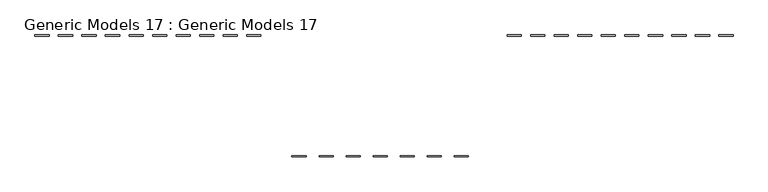
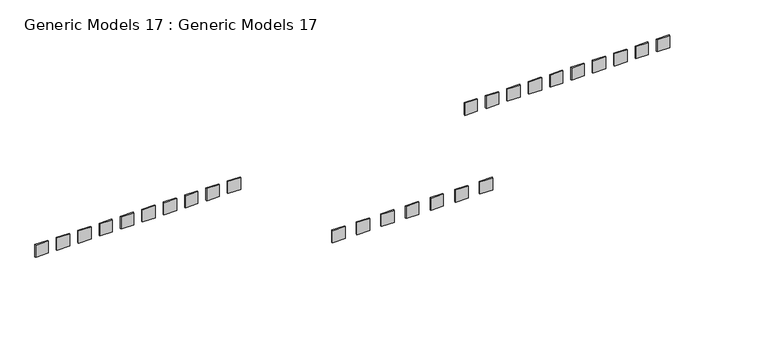
"""IFC4 building model written with IfcOpenShell, lengths in millimetres: proxy geometry, Generic Models 17 : Generic Models 17."""

from ifc_helpers import new_model, si_unit, frame, origin, place, context, project, spatial, polyline, outline, extrude, source, transform, mapped, element, save


def generic_models_17_generic_models_17_0ec560be(model_context):
    return source(origin(), model_context, "Body", "SweptSolid", [
        extrude(outline(polyline([(382.7174924, -8008.8292912), (77.9174924, -8008.8292912), (77.9174924, -7983.4292912), (382.7174924, -7983.4292912), (382.7174924, -8008.8292912)])), frame((0.0, 0.0, 6823.7646282), z_axis=(0.0, 0.0, 1.0), x_axis=(1.0, 0.0, 0.0)), (0.0, 0.0, 1.0), 304.8),
        extrude(outline(polyline([(-201.4825076, -8008.8292912), (-506.2825076, -8008.8292912), (-506.2825076, -7983.4292912), (-201.4825076, -7983.4292912), (-201.4825076, -8008.8292912)])), frame((0.0, 0.0, 6823.7646282), z_axis=(0.0, 0.0, 1.0), x_axis=(1.0, 0.0, 0.0)), (0.0, 0.0, 1.0), 304.8),
        extrude(outline(polyline([(-785.6825076, -8008.8292912), (-1090.4825076, -8008.8292912), (-1090.4825076, -7983.4292912), (-785.6825076, -7983.4292912), (-785.6825076, -8008.8292912)])), frame((0.0, 0.0, 6823.7646282), z_axis=(0.0, 0.0, 1.0), x_axis=(1.0, 0.0, 0.0)), (0.0, 0.0, 1.0), 304.8),
        extrude(outline(polyline([(-1369.8825076, -8008.8292912), (-1674.6825076, -8008.8292912), (-1674.6825076, -7983.4292912), (-1369.8825076, -7983.4292912), (-1369.8825076, -8008.8292912)])), frame((0.0, 0.0, 6823.7646282), z_axis=(0.0, 0.0, 1.0), x_axis=(1.0, 0.0, 0.0)), (0.0, 0.0, 1.0), 304.8),
        extrude(outline(polyline([(-1954.0825076, -8008.8292912), (-2258.8825076, -8008.8292912), (-2258.8825076, -7983.4292912), (-1954.0825076, -7983.4292912), (-1954.0825076, -8008.8292912)])), frame((0.0, 0.0, 6823.7646282), z_axis=(0.0, 0.0, 1.0), x_axis=(1.0, 0.0, 0.0)), (0.0, 0.0, 1.0), 304.8),
        extrude(outline(polyline([(966.9174924, -8008.8292912), (662.1174924, -8008.8292912), (662.1174924, -7983.4292912), (966.9174924, -7983.4292912), (966.9174924, -8008.8292912)])), frame((0.0, 0.0, 6823.7646282), z_axis=(0.0, 0.0, 1.0), x_axis=(1.0, 0.0, 0.0)), (0.0, 0.0, 1.0), 304.8),
        extrude(outline(polyline([(-2538.2825076, -8008.8292912), (-2843.0825076, -8008.8292912), (-2843.0825076, -7983.4292912), (-2538.2825076, -7983.4292912), (-2538.2825076, -8008.8292912)])), frame((0.0, 0.0, 6823.7646282), z_axis=(0.0, 0.0, 1.0), x_axis=(1.0, 0.0, 0.0)), (0.0, 0.0, 1.0), 304.8),
        extrude(outline(polyline([(2617.9174924, -5404.7542653), (2313.1174924, -5404.7542653), (2313.1174924, -5379.3542653), (2617.9174924, -5379.3542653), (2617.9174924, -5404.7542653)])), frame((0.0, 0.0, 6823.7646282), z_axis=(0.0, 0.0, 1.0), x_axis=(1.0, 0.0, 0.0)), (0.0, 0.0, 1.0), 304.8),
        extrude(outline(polyline([(3125.9174924, -5404.7542653), (2821.1174924, -5404.7542653), (2821.1174924, -5379.3542653), (3125.9174924, -5379.3542653), (3125.9174924, -5404.7542653)])), frame((0.0, 0.0, 6823.7646282), z_axis=(0.0, 0.0, 1.0), x_axis=(1.0, 0.0, 0.0)), (0.0, 0.0, 1.0), 304.8),
        extrude(outline(polyline([(3633.9174924, -5404.7542653), (3329.1174924, -5404.7542653), (3329.1174924, -5379.3542653), (3633.9174924, -5379.3542653), (3633.9174924, -5404.7542653)])), frame((0.0, 0.0, 6823.7646282), z_axis=(0.0, 0.0, 1.0), x_axis=(1.0, 0.0, 0.0)), (0.0, 0.0, 1.0), 304.8),
        extrude(outline(polyline([(4141.9174924, -5404.7542653), (3837.1174924, -5404.7542653), (3837.1174924, -5379.3542653), (4141.9174924, -5379.3542653), (4141.9174924, -5404.7542653)])), frame((0.0, 0.0, 6823.7646282), z_axis=(0.0, 0.0, 1.0), x_axis=(1.0, 0.0, 0.0)), (0.0, 0.0, 1.0), 304.8),
        extrude(outline(polyline([(4649.9174924, -5404.7542653), (4345.1174924, -5404.7542653), (4345.1174924, -5379.3542653), (4649.9174924, -5379.3542653), (4649.9174924, -5404.7542653)])), frame((0.0, 0.0, 6823.7646282), z_axis=(0.0, 0.0, 1.0), x_axis=(1.0, 0.0, 0.0)), (0.0, 0.0, 1.0), 304.8),
        extrude(outline(polyline([(5157.9174924, -5404.7542653), (4853.1174924, -5404.7542653), (4853.1174924, -5379.3542653), (5157.9174924, -5379.3542653), (5157.9174924, -5404.7542653)])), frame((0.0, 0.0, 6823.7646282), z_axis=(0.0, 0.0, 1.0), x_axis=(1.0, 0.0, 0.0)), (0.0, 0.0, 1.0), 304.8),
        extrude(outline(polyline([(5665.9174924, -5404.7542653), (5361.1174924, -5404.7542653), (5361.1174924, -5379.3542653), (5665.9174924, -5379.3542653), (5665.9174924, -5404.7542653)])), frame((0.0, 0.0, 6823.7646282), z_axis=(0.0, 0.0, 1.0), x_axis=(1.0, 0.0, 0.0)), (0.0, 0.0, 1.0), 304.8),
        extrude(outline(polyline([(6173.9174924, -5404.7542653), (5869.1174924, -5404.7542653), (5869.1174924, -5379.3542653), (6173.9174924, -5379.3542653), (6173.9174924, -5404.7542653)])), frame((0.0, 0.0, 6823.7646282), z_axis=(0.0, 0.0, 1.0), x_axis=(1.0, 0.0, 0.0)), (0.0, 0.0, 1.0), 304.8),
        extrude(outline(polyline([(2109.9174924, -5404.7542653), (1805.1174924, -5404.7542653), (1805.1174924, -5379.3542653), (2109.9174924, -5379.3542653), (2109.9174924, -5404.7542653)])), frame((0.0, 0.0, 6823.7646282), z_axis=(0.0, 0.0, 1.0), x_axis=(1.0, 0.0, 0.0)), (0.0, 0.0, 1.0), 304.8),
        extrude(outline(polyline([(6681.9174924, -5404.7542653), (6377.1174924, -5404.7542653), (6377.1174924, -5379.3542653), (6681.9174924, -5379.3542653), (6681.9174924, -5404.7542653)])), frame((0.0, 0.0, 6823.7646282), z_axis=(0.0, 0.0, 1.0), x_axis=(1.0, 0.0, 0.0)), (0.0, 0.0, 1.0), 304.8),
        extrude(outline(polyline([(-4024.1825076, -5404.7542653), (-4328.9825076, -5404.7542653), (-4328.9825076, -5379.3542653), (-4024.1825076, -5379.3542653), (-4024.1825076, -5404.7542653)])), frame((0.0, 0.0, 6823.7646282), z_axis=(0.0, 0.0, 1.0), x_axis=(1.0, 0.0, 0.0)), (0.0, 0.0, 1.0), 304.8),
        extrude(outline(polyline([(-4532.1825076, -5404.7542653), (-4836.9825076, -5404.7542653), (-4836.9825076, -5379.3542653), (-4532.1825076, -5379.3542653), (-4532.1825076, -5404.7542653)])), frame((0.0, 0.0, 6823.7646282), z_axis=(0.0, 0.0, 1.0), x_axis=(1.0, 0.0, 0.0)), (0.0, 0.0, 1.0), 304.8),
        extrude(outline(polyline([(-5040.1825076, -5404.7542653), (-5344.9825076, -5404.7542653), (-5344.9825076, -5379.3542653), (-5040.1825076, -5379.3542653), (-5040.1825076, -5404.7542653)])), frame((0.0, 0.0, 6823.7646282), z_axis=(0.0, 0.0, 1.0), x_axis=(1.0, 0.0, 0.0)), (0.0, 0.0, 1.0), 304.8),
        extrude(outline(polyline([(-5548.1825076, -5404.7542653), (-5852.9825076, -5404.7542653), (-5852.9825076, -5379.3542653), (-5548.1825076, -5379.3542653), (-5548.1825076, -5404.7542653)])), frame((0.0, 0.0, 6823.7646282), z_axis=(0.0, 0.0, 1.0), x_axis=(1.0, 0.0, 0.0)), (0.0, 0.0, 1.0), 304.8),
        extrude(outline(polyline([(-6056.1825076, -5404.7542653), (-6360.9825076, -5404.7542653), (-6360.9825076, -5379.3542653), (-6056.1825076, -5379.3542653), (-6056.1825076, -5404.7542653)])), frame((0.0, 0.0, 6823.7646282), z_axis=(0.0, 0.0, 1.0), x_axis=(1.0, 0.0, 0.0)), (0.0, 0.0, 1.0), 304.8),
        extrude(outline(polyline([(-6564.1825076, -5404.7542653), (-6868.9825076, -5404.7542653), (-6868.9825076, -5379.3542653), (-6564.1825076, -5379.3542653), (-6564.1825076, -5404.7542653)])), frame((0.0, 0.0, 6823.7646282), z_axis=(0.0, 0.0, 1.0), x_axis=(1.0, 0.0, 0.0)), (0.0, 0.0, 1.0), 304.8),
        extrude(outline(polyline([(-7072.1825076, -5404.7542653), (-7376.9825076, -5404.7542653), (-7376.9825076, -5379.3542653), (-7072.1825076, -5379.3542653), (-7072.1825076, -5404.7542653)])), frame((0.0, 0.0, 6823.7646282), z_axis=(0.0, 0.0, 1.0), x_axis=(1.0, 0.0, 0.0)), (0.0, 0.0, 1.0), 304.8),
        extrude(outline(polyline([(-7580.1825076, -5404.7542653), (-7884.9825076, -5404.7542653), (-7884.9825076, -5379.3542653), (-7580.1825076, -5379.3542653), (-7580.1825076, -5404.7542653)])), frame((0.0, 0.0, 6823.7646282), z_axis=(0.0, 0.0, 1.0), x_axis=(1.0, 0.0, 0.0)), (0.0, 0.0, 1.0), 304.8),
        extrude(outline(polyline([(-3516.1825076, -5404.7542653), (-3820.9825076, -5404.7542653), (-3820.9825076, -5379.3542653), (-3516.1825076, -5379.3542653), (-3516.1825076, -5404.7542653)])), frame((0.0, 0.0, 6823.7646282), z_axis=(0.0, 0.0, 1.0), x_axis=(1.0, 0.0, 0.0)), (0.0, 0.0, 1.0), 304.8),
        extrude(outline(polyline([(-8088.1825076, -5404.7542653), (-8392.9825076, -5404.7542653), (-8392.9825076, -5379.3542653), (-8088.1825076, -5379.3542653), (-8088.1825076, -5404.7542653)])), frame((0.0, 0.0, 6823.7646282), z_axis=(0.0, 0.0, 1.0), x_axis=(1.0, 0.0, 0.0)), (0.0, 0.0, 1.0), 304.8),
    ])


if __name__ == "__main__":
    model = new_model("IFC4")
    model_context = context("Model", 3, world=origin())
    ifc_project = project(units=[si_unit("LENGTHUNIT", "METRE", prefix="MILLI")], contexts=[model_context])
    site = spatial("IfcSite", under=ifc_project)
    building = spatial("IfcBuilding", under=site)
    placement = place(None, origin())
    generic_models_17_generic_models_17_shape = generic_models_17_generic_models_17_0ec560be(model_context)
    element("IfcBuildingElementProxy", 1, Name="Generic Models 17 : Generic Models 17", ObjectType="Generic Models 17 : Generic Models 17", at=placement, inside=building, context=model_context, shape_type="MappedRepresentation", body=[
        mapped(generic_models_17_generic_models_17_shape, transform((0.0, 0.0, 0.0), x_axis=(1.0, 0.0, 0.0), y_axis=(0.0, 1.0, 0.0), z_axis=(0.0, 0.0, 1.0))),
    ])
    save(model, "model.ifc")
